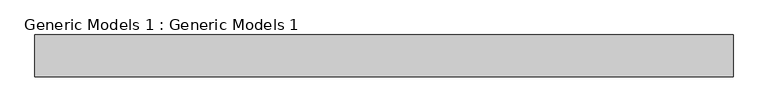
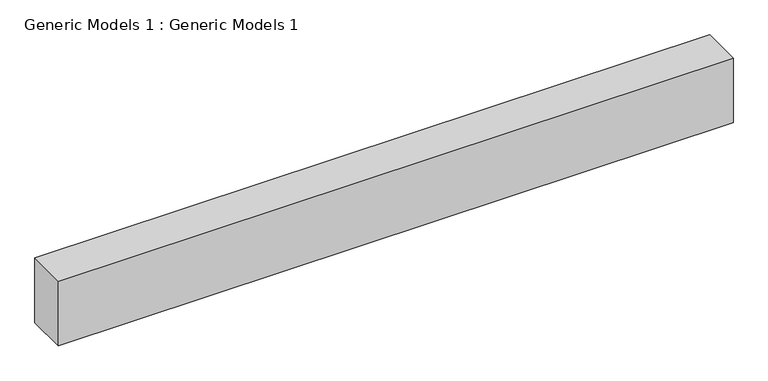
"""IFC4 building model written with IfcOpenShell, lengths in millimetres: proxy geometry, Generic Models 1 : Generic Models 1."""

from ifc_helpers import new_model, si_unit, frame, origin, place, context, project, spatial, polyline, outline, extrude, source, transform, mapped, element, save


def generic_models_1_generic_models_1_53319598(model_context):
    return source(origin(), model_context, "Body", "SweptSolid", [
        extrude(outline(polyline([(-4601.1678816, 1946.1030358), (-7611.0678816, 1946.1030358), (-7611.0678816, 2126.5115792), (-4601.1678816, 2126.5115792), (-4601.1678816, 1946.1030358)])), frame((0.0, 0.0, 5943.6), z_axis=(0.0, 0.0, 1.0), x_axis=(1.0, 0.0, 0.0)), (0.0, 0.0, 1.0), 304.8),
    ])


if __name__ == "__main__":
    model = new_model("IFC4")
    model_context = context("Model", 3, world=origin())
    ifc_project = project(units=[si_unit("LENGTHUNIT", "METRE", prefix="MILLI")], contexts=[model_context])
    site = spatial("IfcSite", under=ifc_project)
    building = spatial("IfcBuilding", under=site)
    placement = place(None, origin())
    generic_models_1_generic_models_1_shape = generic_models_1_generic_models_1_53319598(model_context)
    element("IfcBuildingElementProxy", 1, Name="Generic Models 1 : Generic Models 1", ObjectType="Generic Models 1 : Generic Models 1", at=placement, inside=building, context=model_context, shape_type="MappedRepresentation", body=[
        mapped(generic_models_1_generic_models_1_shape, transform((0.0, 0.0, 0.0), x_axis=(1.0, 0.0, 0.0), y_axis=(0.0, 1.0, 0.0), z_axis=(0.0, 0.0, 1.0))),
    ])
    save(model, "model.ifc")

# Revit data of these elements
# Element 1 (IfcBuildingElementProxy, "Generic Models 1 : Generic Models 1")
#   Materials on its faces: "wall paint"
# Materials
#   "wall paint": class "Generic", colour RGB 120 120 120, transparency 0, Cost = 0
